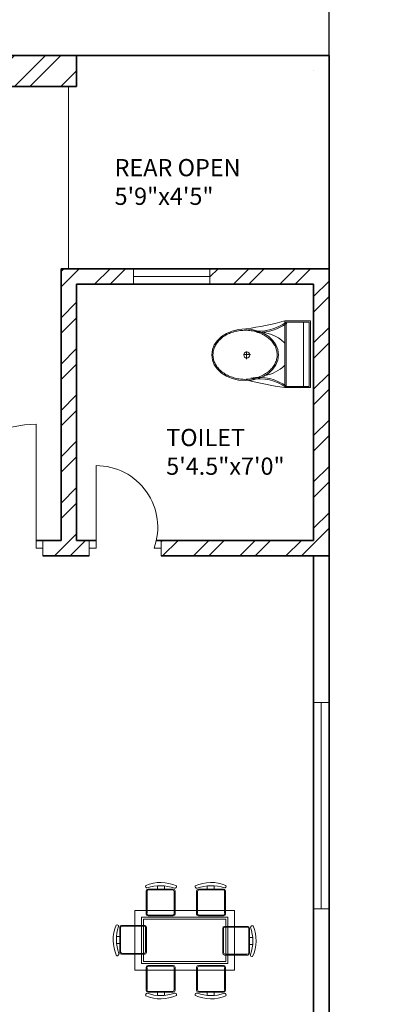
# Model space of a CAD drawing. Units: inches. Extents: x 1850 to 3445, y 1558 to 2756.
# Tile 4 of 13: x 2195 to 2304, y 1940 to 2227. Entities that reach past the tile are written whole.
import ezdxf

# ---------------------------------------------------------------- set-up
doc = ezdxf.new("R2010")
doc.units = ezdxf.units.IN
for name, color, linetype, lineweight in [('A-ANNO-DIMS', 2, 'Continuous', 18), ('A-AREA-IDEN', 7, 'Continuous', 18), ('A-DOOR', 3, 'Continuous', 18), ('A-FLOR-FIXT', 9, 'Continuous', 18), ('A-FURN', 8, 'Continuous', 13), ('A-GLAZ', 4, 'Continuous', 18), ('A-WALL', 7, 'Continuous', 35), ('A-WALL-PATT', 252, 'Continuous', 13)]:
    doc.layers.add(name, color=color, linetype=linetype, lineweight=lineweight)
doc.styles.get("Standard").update_dxf_attribs({"font": 'arial.ttf'})
doc.dimstyles.get("Standard").update_dxf_attribs({"dimtxt": 0.18, "dimasz": 0.18, "dimexe": 0.18, "dimexo": 0.0625, "dimgap": 0.09, "dimtad": 0, "dimtih": 1, "dimtoh": 1, "dimdec": 4, "dimzin": 0, "dimdsep": 46, "dimtxsty": 'Standard', "dimcen": 0.09, "dimadec": 0, "dimazin": 0, "dimtfac": 1, "dimtdec": 4, "dimtofl": 0, "dimtmove": 0, "dimatfit": 3, "dimfxl": 1, "dimtolj": 1, "dimtzin": 0, "dimarcsym": 0})

# ---------------------------------------------------------------- blocks, each defined once
blk = doc.blocks.new('A$C31115884')
for p, q in [((283.1, 497.7), (223.4, 497.7)), ((257.5, 466.4), (257.5, 523.2)), ((0, 200), (0, 0)), ((520, 200), (0, 200)), ((10, 190), (10, 10)), ((510, 190), (10, 190)), ((510, 10), (510, 190)), ((520, 0), (520, 200)), ((510, 54.5), (0, 54.5)), ((10, 10), (510, 10)), ((0, 0), (520, 0))]:
    blk.add_line(p, q)
blk.add_circle((255.6, 496.4), 23.6)
for centre, radius, start, end in [((2777.7, -204.6), 2807, 165.4549, 171.71327), ((-294.5, 403.3), 364.7, 324.20913, 9.34987), ((-294.5, 403.3), 374.7, 324.20913, 9.34987), ((805.8, 403.3), 364.7, 170.65013, 215.79087), ((3237, 905), 2807, 188.28673, 194.5451), ((139.5, 406.2), 293.5, 315.84364, 2.65635), ((805.8, 403.3), 374.7, 179.20365, 215.79087), ((383.6, 406.2), 293.5, 190.27735, 224.15636)]:
    blk.add_arc(centre, radius, start, end)
blk.add_ellipse((256.2, 509.9), major_axis=(0, -260.7), ratio=0.772727)
blk.add_open_spline([(256.2, 259.2), (263.1, 259.2), (270, 259.7), (287.8, 262.3), (298.7, 265.1), (319.9, 273.1), (330.2, 278.4), (350.1, 291.1), (359.7, 298.7), (377.7, 315.9), (386.2, 325.5), (401.7, 346.6), (408.8, 358.1), (421.3, 382.5), (426.8, 395.5), (435.9, 422.4), (439.5, 436.4), (444.8, 465.1), (446.5, 479.7), (447.9, 509.2), (447.6, 524), (445, 553.3), (442.7, 567.8), (436.3, 596), (432.1, 609.7), (421.9, 636), (416, 648.6), (402.5, 672.1), (395, 683), (378.6, 703), (369.8, 712.1), (351.1, 728), (341.3, 734.8), (320.9, 746.2), (310.4, 750.7), (288.9, 757.3), (278, 759.4), (256, 761), (245, 760.6), (223.1, 757.2), (212.3, 754.3), (191.1, 746.1), (180.8, 740.7), (160.9, 727.8), (151.4, 720.1), (133.5, 702.7), (125.1, 693), (109.6, 671.7), (102.6, 660.2), (90.2, 635.7), (84.9, 622.7), (76, 595.6), (72.4, 581.6), (67.2, 552.9), (65.6, 538.2), (64.4, 508.8), (64.8, 494), (67.5, 464.7), (69.9, 450.2), (76.6, 422), (80.8, 408.3), (91.1, 382.2), (97.2, 369.7), (110.8, 346.3), (118.4, 335.4), (134.8, 315.6), (143.7, 306.7), (162.4, 290.9), (172.3, 284.2), (192.8, 273), (203.3, 268.6), (224.8, 262.2), (235.8, 260.2), (249.9, 259.3), (253, 259.2), (256.2, 259.2)], degree=3, knots=[0, 0, 0, 0, 0.110105, 0.110105, 0.285049, 0.285049, 0.459994, 0.459994, 0.634938, 0.634938, 0.809882, 0.809882, 0.984827, 0.984827, 1.159771, 1.159771, 1.334715, 1.334715, 1.50966, 1.50966, 1.684604, 1.684604, 1.859549, 1.859549, 2.034493, 2.034493, 2.209437, 2.209437, 2.384382, 2.384382, 2.559326, 2.559326, 2.73427, 2.73427, 2.909215, 2.909215, 3.084159, 3.084159, 3.259103, 3.259103, 3.434048, 3.434048, 3.608992, 3.608992, 3.783936, 3.783936, 3.958881, 3.958881, 4.133825, 4.133825, 4.30877, 4.30877, 4.483714, 4.483714, 4.658658, 4.658658, 4.833603, 4.833603, 5.008547, 5.008547, 5.183491, 5.183491, 5.358436, 5.358436, 5.53338, 5.53338, 5.708324, 5.708324, 5.883269, 5.883269, 6.058213, 6.058213, 6.233158, 6.233158, 6.283185, 6.283185, 6.283185, 6.283185])
blk = doc.blocks.new('WIN-60-W4_5')
for p, q in [((0, 60), (4.5, 60)), ((4.5, 60), (2.25, 60)), ((2.25, 60), (2.25, 0)), ((2.25, 0), (0, 0)), ((0, 0), (4.5, 0))]:
    blk.add_line(p, q)
blk = doc.blocks.new('WIN-BATH-GROUND')
for p, q in [((0, 0), (0, 4.5)), ((22.27, 2.25), (22.27, 4.5)), ((22.27, 4.5), (22.27, 0)), ((0, 2.25), (22.27, 2.25))]:
    blk.add_line(p, q)
blk = doc.blocks.new('DOOR-BATH-GROUND')
for p, q in [((2, 2.25), (2, 26.25)), ((0, 4.5), (0, 0)), ((20.9, 4.5), (20.9, 0)), ((0, 0), (0, 2.25)), ((0, 2.25), (2, 2.25)), ((20.9, 2.25), (18.9, 2.25)), ((20.9, 0), (20.9, 2.25))]:
    blk.add_line(p, q)
blk.add_arc((2, 8.3), 17.95, 340.2941, 90)
blk = doc.blocks.new('DOOR-BED-GROUND')
for p, q in [((31.38, 2.25), (31.38, 38.25)), ((0, 4.5), (0, 0)), ((33.38, 4.5), (33.38, 0)), ((0, 0), (0, 2.25)), ((0, 2.25), (2, 2.25)), ((33.38, 2.25), (31.38, 2.25)), ((33.38, 0), (33.38, 2.25))]:
    blk.add_line(p, q)
blk.add_arc((31.38, 8.26), 29.99, 90, 191.5706)
blk = doc.blocks.new('*D80')
at = {"layer": 'A-ANNO-DIMS', "color": 0, "lineweight": -2, "transparency": 16777216}
for p, q in [((2040.27, 2216.25), (2040.27, 2244.61)), ((2040.45, 2244.43), (2162.48, 2244.43)), ((2285.09, 2244.43), (2163.06, 2244.43)), ((2285.27, 2216.25), (2285.27, 2244.61))]:
    blk.add_line(p, q, dxfattribs=at)
at = {"layer": 'A-ANNO-DIMS', "color": 0, "transparency": 16777216}
for points in [[(2040.45, 2244.46), (2040.45, 2244.4), (2040.27, 2244.43)], [(2285.09, 2244.46), (2285.09, 2244.4), (2285.27, 2244.43)]]:
    blk.add_solid(points, dxfattribs=at)
at = {"layer": 'Defpoints', "color": 0, "transparency": 16777216}
for p in [(2285.27, 2244.43), (2040.27, 2216.18), (2285.27, 2216.18)]:
    blk.add_point(p, dxfattribs=at)
at = {"layer": 'A-ANNO-DIMS', "color": 0, "transparency": 16777216, "insert": (2162.77, 2244.43), "char_height": 0.18, "attachment_point": 5}
blk.add_mtext('\\A1;245', dxfattribs=at)

msp = doc.modelspace()

# ---------------------------------------------------------------- hatches: boundary and pattern name
at = {"layer": 'A-WALL-PATT'}
h = msp.add_hatch(dxfattribs=at)
h.set_pattern_fill('ANSI32', color=256)
h.paths.add_polyline_path([(2519.5556, 1907.3936), (2523.9987, 1907.3936), (2523.9987, 1916.3936), (2519.5556, 1916.3936), (2515.0556, 1916.3936), (2510.5556, 1916.3936), (2510.5556, 1907.3936), (2515.0556, 1907.3936), (2515.0556, 1742.1843), (2515.0556, 1737.6843), (2596.0556, 1737.6843), (2596.0556, 1976.4962), (2591.5556, 1976.4962), (2591.5556, 1916.3936), (2561.2666, 1916.3936), (2561.2666, 1907.3936), (2591.5556, 1907.3936), (2591.5556, 1746.6843), (2519.5556, 1746.6843)])
h.paths.add_polyline_path([(2076.6481, 2211.6843), (2076.6481, 2216.1843), (2040.2715, 2216.1843), (2040.2715, 2175.83), (2044.7715, 2175.83), (2049.2715, 2175.83), (2049.2715, 2207.1843), (2076.6481, 2207.1843)])
h.paths.add_polyline_path([(2211.7715, 2216.1843), (2136.6481, 2216.1843), (2136.6481, 2207.1843), (2211.7715, 2207.1843)])
h.paths.add_polyline_path([(2285.2715, 2154.1843), (2250.6169, 2154.1843), (2250.6169, 2149.6843), (2280.7715, 2149.6843), (2280.7715, 2075.1843), (2236.3632, 2075.1843), (2236.3632, 2070.6843), (2285.2715, 2070.6843)])
h.paths.add_polyline_path([(2228.3485, 2154.1843), (2207.2715, 2154.1843), (2207.2715, 2075.1843), (2201.9819, 2075.1843), (2201.9819, 2070.6843), (2215.4663, 2070.6843), (2215.4663, 2072.9343), (2215.4663, 2075.1843), (2211.7715, 2075.1843), (2211.7715, 2149.6843), (2228.3485, 2149.6843)])
h.paths.add_polyline_path([(2049.2715, 2115.83), (2040.2715, 2115.83), (2040.2715, 2042.8465), (2049.2715, 2042.8465), (2049.2715, 2070.6843), (2168.6057, 2070.6843), (2168.6057, 2072.9343), (2168.6057, 2075.1843), (2049.2715, 2075.1843)])
h.paths.add_polyline_path([(2049.2715, 1982.8465), (2040.2715, 1982.8465), (2040.2715, 1910.2175), (2060.9481, 1910.2175), (2060.9481, 1914.7175), (2060.9481, 1919.2175), (2049.2715, 1919.2175)])
h.paths.add_polyline_path([(2132.4938, 1919.2175), (2108.9481, 1919.2175), (2108.9481, 1910.2175), (2132.4938, 1910.2175), (2132.4938, 1914.6749)])
h.paths.add_polyline_path([(2178.7715, 1938.6843), (2169.7715, 1938.6843), (2169.7715, 1919.2175), (2163.687, 1919.2175), (2163.687, 1910.2175), (2169.7715, 1910.2175), (2169.7715, 1854.6843), (2169.7715, 1845.6843), (2196.1287, 1845.6843), (2196.1287, 1850.1843), (2196.1287, 1854.6843), (2178.7715, 1854.6843)])
h.paths.add_polyline_path([(2049.2715, 1910.2175), (2040.2715, 1910.2175), (2040.2715, 1745.6843), (2049.2715, 1745.6843)])
h.paths.add_polyline_path([(2146.8861, 1766.7204), (2159.0894, 1766.7204), (2159.0894, 1777.0239), (2146.8861, 1777.0239)], flags=9)
h.paths.add_polyline_path([(2183.4664, 1798.4016), (2226.7338, 1798.4016), (2226.7338, 1817.0589), (2183.4664, 1817.0589)], flags=9)
h.paths.add_polyline_path([(2070.863, 1867.537), (2109.9796, 1867.537), (2109.9796, 1886.1943), (2070.863, 1886.1943)], flags=9)

# ---------------------------------------------------------------- linework, layer by layer
at = {"layer": 'A-FURN'}
for points in [[(2232.3545, 1974.0971, -0.17580919), (2240.2562, 1974.0373, 0.57839206), (2240.8548, 1974.6955, 0.21452438), (2231.9355, 1974.8152, 0.55201397), (2232.3545, 1974.0971, -0.06507904)], [(2232.3545, 1974.0968, -0.17580919), (2240.2562, 1974.037, 0.57839206), (2240.8548, 1974.6952, 0.21452438), (2231.9355, 1974.8149, 0.55201397), (2232.3545, 1974.0968, -0.06507904)], [(2246.9084, 1974.0373, -0.57839206), (2246.3098, 1974.6955, -0.21452438), (2255.2292, 1974.8152, -0.55201397), (2254.8101, 1974.0971, 0.1758092), (2246.9084, 1974.0373)], [(2246.9084, 1974.037, -0.57839206), (2246.3098, 1974.6952, -0.21452438), (2255.2292, 1974.8149, -0.55201397), (2254.8101, 1974.0968, 0.1758092), (2246.9084, 1974.037)], [(2239.921, 1973.78), (2232.5853, 1973.78, 0.41421356), (2232.0721, 1973.2668), (2232.0721, 1966.5217, 0.41421356), (2232.5853, 1966.0085), (2239.921, 1966.0085, 0.41421356), (2240.4342, 1966.5217), (2240.4342, 1973.2668, 0.41421356), (2239.921, 1973.78)], [(2239.921, 1973.7797), (2232.5853, 1973.7797, 0.41421356), (2232.0721, 1973.2665), (2232.0721, 1966.5214, 0.41421356), (2232.5853, 1966.0082), (2239.921, 1966.0082, 0.41421356), (2240.4342, 1966.5214), (2240.4342, 1973.2665, 0.41421356), (2239.921, 1973.7797)], [(2237.3443, 1973.78), (2237.3443, 1974.7077, -0.06475861)], [(2237.3443, 1973.7797), (2237.3443, 1974.7074, -0.06475861)], [(2254.5793, 1973.78, -0.41421356), (2255.0925, 1973.2668), (2255.0925, 1966.5217, -0.41421356), (2254.5793, 1966.0085), (2247.2437, 1966.0085, -0.41421356), (2246.7304, 1966.5217), (2246.7304, 1973.2668, -0.41421356), (2247.2437, 1973.78), (2254.5793, 1973.78)], [(2254.5793, 1973.7797, -0.41421356), (2255.0926, 1973.2665), (2255.0926, 1966.5214, -0.41421356), (2254.5793, 1966.0082), (2247.2437, 1966.0082, -0.41421356), (2246.7305, 1966.5214), (2246.7305, 1973.2665, -0.41421356), (2247.2437, 1973.7797), (2254.5793, 1973.7797)], [(2249.8203, 1973.78), (2249.8203, 1974.7077, 0.06475861)], [(2249.8203, 1973.7797), (2249.8203, 1974.7074, 0.06475861)], [(2224.0878, 1955.0157, -0.57839206), (2223.4296, 1954.4171, -0.21452438), (2223.3099, 1963.3364, -0.55201397), (2224.028, 1962.9174, 0.17580937), (2224.0878, 1955.0157)], [(2224.0878, 1955.0154, -0.57839206), (2223.4296, 1954.4168, -0.21452438), (2223.3099, 1963.3361, -0.55201397), (2224.028, 1962.9171, 0.17580937), (2224.0878, 1955.0154)], [(2224.3451, 1962.6866, -0.41421356), (2224.8583, 1963.1998), (2231.6033, 1963.1998, -0.41421356), (2232.1165, 1962.6866), (2232.1165, 1955.3509, -0.41421356), (2231.6033, 1954.8377), (2224.8583, 1954.8377, -0.41421356), (2224.3451, 1955.3509), (2224.3451, 1962.6866)], [(2224.3451, 1962.6863, -0.41421356), (2224.8583, 1963.1995), (2231.6033, 1963.1995, -0.41421356), (2232.1166, 1962.6863), (2232.1166, 1955.3506, -0.41421356), (2231.6033, 1954.8374), (2224.8583, 1954.8374, -0.41421356), (2224.3451, 1955.3506), (2224.3451, 1962.6863)], [(2262.1204, 1962.4354, 0.41421356), (2261.6072, 1962.9486), (2254.8622, 1962.9486, 0.41421356), (2254.349, 1962.4354), (2254.349, 1955.0997, 0.41421356), (2254.8622, 1954.5865), (2261.6072, 1954.5865, 0.41421356), (2262.1204, 1955.0997), (2262.1204, 1962.4354)], [(2262.1204, 1962.4351, 0.41421356), (2261.6072, 1962.9483), (2254.8622, 1962.9483, 0.41421356), (2254.349, 1962.4351), (2254.349, 1955.0994, 0.41421356), (2254.8622, 1954.5862), (2261.6072, 1954.5862, 0.41421356), (2262.1204, 1955.0994), (2262.1204, 1962.4351)], [(2262.4375, 1962.6662, -0.17580919), (2262.3777, 1954.7645, 0.57839206), (2263.0359, 1954.1658, 0.21452438), (2263.1556, 1963.0852, 0.55201397), (2262.4375, 1962.6662, -0.06507904)], [(2262.4375, 1962.6659, -0.17580919), (2262.3777, 1954.7642, 0.57839206), (2263.0359, 1954.1655, 0.21452438), (2263.1556, 1963.0849, 0.55201397), (2262.4375, 1962.6659, -0.06507904)], [(2224.3451, 1957.9276), (2223.4174, 1957.9276, 0.06475861)], [(2224.3451, 1957.9273), (2223.4174, 1957.9273, 0.06475861)], [(2262.1204, 1957.6764), (2263.0481, 1957.6764, -0.06475861)], [(2262.1204, 1957.676), (2263.0481, 1957.676, -0.06475861)], [(2239.921, 1943.7967), (2232.5853, 1943.7967, -0.41421356), (2232.0721, 1944.31), (2232.0721, 1951.055, -0.41421356), (2232.5853, 1951.5682), (2239.921, 1951.5682, -0.41421356), (2240.4342, 1951.055), (2240.4342, 1944.31, -0.41421356), (2239.921, 1943.7967)], [(2239.921, 1943.7964), (2232.5853, 1943.7964, -0.41421356), (2232.0721, 1944.3097), (2232.0721, 1951.0547, -0.41421356), (2232.5853, 1951.5679), (2239.921, 1951.5679, -0.41421356), (2240.4342, 1951.0547), (2240.4342, 1944.3097, -0.41421356), (2239.921, 1943.7964)], [(2254.5793, 1943.7967, 0.41421356), (2255.0925, 1944.31), (2255.0925, 1951.055, 0.41421356), (2254.5793, 1951.5682), (2247.2437, 1951.5682, 0.41421356), (2246.7304, 1951.055), (2246.7304, 1944.31, 0.41421356), (2247.2437, 1943.7967), (2254.5793, 1943.7967)], [(2254.5793, 1943.7964, 0.41421356), (2255.0926, 1944.3097), (2255.0926, 1951.0547, 0.41421356), (2254.5793, 1951.5679), (2247.2437, 1951.5679, 0.41421356), (2246.7305, 1951.0547), (2246.7305, 1944.3097, 0.41421356), (2247.2437, 1943.7964), (2254.5793, 1943.7964)], [(2240.2562, 1943.5394, -0.57839206), (2240.8548, 1942.8812, -0.21452438), (2231.9355, 1942.7615, -0.55201397), (2232.3545, 1943.4796, 0.17580929), (2240.2562, 1943.5394)], [(2240.2562, 1943.5391, -0.57839206), (2240.8548, 1942.8809, -0.21452438), (2231.9355, 1942.7612, -0.55201397), (2232.3545, 1943.4793, 0.17580929), (2240.2562, 1943.5391)], [(2237.3443, 1943.7967), (2237.3443, 1942.869, 0.06475861)], [(2237.3443, 1943.7964), (2237.3443, 1942.8687, 0.06475861)], [(2254.8101, 1943.4796, -0.17580928), (2246.9084, 1943.5394, 0.57839206), (2246.3098, 1942.8812, 0.21452438), (2255.2292, 1942.7615, 0.55201397), (2254.8101, 1943.4796, -0.06507904)], [(2254.8101, 1943.4793, -0.17580928), (2246.9084, 1943.5391, 0.57839206), (2246.3098, 1942.8809, 0.21452438), (2255.2292, 1942.7612, 0.55201397), (2254.8101, 1943.4793, -0.06507904)], [(2249.8203, 1943.7967), (2249.8203, 1942.869, -0.06475861)], [(2249.8203, 1943.7964), (2249.8203, 1942.8687, -0.06475861)]]:
    msp.add_lwpolyline(points, format="xyb", dxfattribs=at)
for points in [[(2232.5884, 1973.5488), (2239.6898, 1973.5488, -0.41421356), (2240.203, 1973.0356), (2240.203, 1966.753, -0.41421356), (2239.6898, 1966.2397), (2232.5884, 1966.2397, -0.51206948), (2232.3033, 1966.753), (2232.3033, 1973.0356, -0.51206948)], [(2232.5884, 1973.5485), (2239.6898, 1973.5485, -0.41421356), (2240.203, 1973.0352), (2240.203, 1966.7526, -0.41421356), (2239.6898, 1966.2394), (2232.5884, 1966.2394, -0.51206948), (2232.3033, 1966.7526), (2232.3033, 1973.0352, -0.51206948)], [(2254.5762, 1973.5488), (2247.4749, 1973.5488, 0.41421356), (2246.9617, 1973.0356), (2246.9617, 1966.753, 0.41421356), (2247.4749, 1966.2397), (2254.5762, 1966.2397, 0.51206948), (2254.8613, 1966.753), (2254.8613, 1973.0356, 0.51206948)], [(2254.5762, 1973.5485), (2247.4749, 1973.5485, 0.41421356), (2246.9617, 1973.0352), (2246.9617, 1966.7526, 0.41421356), (2247.4749, 1966.2394), (2254.5762, 1966.2394, 0.51206948), (2254.8614, 1966.7526), (2254.8614, 1973.0352, 0.51206948)], [(2224.5763, 1962.6835), (2224.5763, 1955.5821, 0.41421356), (2225.0895, 1955.0689), (2231.3721, 1955.0689, 0.41421356), (2231.8853, 1955.5821), (2231.8853, 1962.6835, 0.51206948), (2231.3721, 1962.9686), (2225.0895, 1962.9686, 0.51206948)], [(2224.5763, 1962.6832), (2224.5763, 1955.5818, 0.41421356), (2225.0895, 1955.0686), (2231.3721, 1955.0686, 0.41421356), (2231.8854, 1955.5818), (2231.8854, 1962.6832, 0.51206948), (2231.3721, 1962.9683), (2225.0895, 1962.9683, 0.51206948)], [(2261.8892, 1962.4323), (2261.8892, 1955.3309, -0.41421356), (2261.376, 1954.8177), (2255.0934, 1954.8177, -0.41421356), (2254.5802, 1955.3309), (2254.5802, 1962.4323, -0.51206948), (2255.0934, 1962.7174), (2261.376, 1962.7174, -0.51206948)], [(2261.8892, 1962.432), (2261.8892, 1955.3306, -0.41421356), (2261.376, 1954.8174), (2255.0934, 1954.8174, -0.41421356), (2254.5802, 1955.3306), (2254.5802, 1962.432, -0.51206948), (2255.0934, 1962.7171), (2261.376, 1962.7171, -0.51206948)], [(2232.5884, 1944.028), (2239.6898, 1944.028, 0.41421356), (2240.203, 1944.5412), (2240.203, 1950.8238, 0.41421356), (2239.6898, 1951.337), (2232.5884, 1951.337, 0.51206948), (2232.3033, 1950.8238), (2232.3033, 1944.5412, 0.51206948)], [(2232.5884, 1944.0276), (2239.6898, 1944.0276, 0.41421356), (2240.203, 1944.5409), (2240.203, 1950.8235, 0.41421356), (2239.6898, 1951.3367), (2232.5884, 1951.3367, 0.51206948), (2232.3033, 1950.8235), (2232.3033, 1944.5409, 0.51206948)], [(2254.5762, 1944.028), (2247.4749, 1944.028, -0.41421356), (2246.9617, 1944.5412), (2246.9617, 1950.8238, -0.41421356), (2247.4749, 1951.337), (2254.5762, 1951.337, -0.51206948), (2254.8613, 1950.8238), (2254.8613, 1944.5412, -0.51206948)], [(2254.5762, 1944.0276), (2247.4749, 1944.0276, -0.41421356), (2246.9617, 1944.5409), (2246.9617, 1950.8235, -0.41421356), (2247.4749, 1951.3367), (2254.5762, 1951.3367, -0.51206948), (2254.8614, 1950.8235), (2254.8614, 1944.5409, -0.51206948)]]:
    msp.add_lwpolyline(points, format="xyb", close=True, dxfattribs=at)
for points in [[(2235.291, 1974.7246), (2235.291, 1973.78)], [(2235.291, 1974.7243), (2235.291, 1973.7797)], [(2251.8737, 1974.7246), (2251.8737, 1973.78)], [(2251.8737, 1974.7243), (2251.8737, 1973.7797)], [(2223.4005, 1959.9809), (2224.3451, 1959.9809)], [(2223.4005, 1959.9806), (2224.3451, 1959.9806)], [(2263.065, 1959.7297), (2262.1204, 1959.7297)], [(2263.065, 1959.7294), (2262.1204, 1959.7294)], [(2235.291, 1942.8521), (2235.291, 1943.7967)], [(2235.291, 1942.8518), (2235.291, 1943.7964)], [(2251.8737, 1942.8521), (2251.8737, 1943.7967)], [(2251.8737, 1942.8518), (2251.8737, 1943.7964)]]:
    msp.add_lwpolyline(points, dxfattribs=at)
for points in [[(2228.7662, 1967.5848), (2257.7769, 1967.5848), (2257.7769, 1950.1784), (2228.7662, 1950.1784)], [(2228.7662, 1967.5845), (2257.7769, 1967.5845), (2257.7769, 1950.1781), (2228.7662, 1950.1781)], [(2230.7002, 1965.6508), (2255.8429, 1965.6508), (2255.8429, 1952.1124), (2230.7002, 1952.1124)], [(2230.7002, 1965.6504), (2255.8429, 1965.6504), (2255.8429, 1952.1121), (2230.7002, 1952.1121)], [(2231.2804, 1965.0705), (2255.2627, 1965.0705), (2255.2627, 1952.6926), (2231.2804, 1952.6926)], [(2231.2805, 1965.0702), (2255.2627, 1965.0702), (2255.2627, 1952.6923), (2231.2805, 1952.6923)]]:
    msp.add_lwpolyline(points, close=True, dxfattribs=at)
at = {"layer": 'A-GLAZ'}
msp.add_line((2209.4518, 2207.1843), (2209.4518, 2154.1843), dxfattribs=at)
at = {"layer": 'A-WALL'}
for p, q in [((2040.2715, 2216.1843), (2285.2715, 2216.1843)), ((2211.7715, 2216.1843), (2211.7715, 2207.1843)), ((2285.2715, 2207.1843), (2285.2715, 2216.1843)), ((2280.7444, 2211.8893), (2280.7444, 2211.8893)), ((2049.2715, 2207.1843), (2211.7715, 2207.1843)), ((2285.2715, 2207.1843), (2285.2715, 1745.6843)), ((2207.2715, 2154.1843), (2207.2715, 2075.1843)), ((2207.2715, 2154.1843), (2285.2715, 2154.1843)), ((2211.7715, 2149.6843), (2280.7715, 2149.6843)), ((2211.7715, 2149.6843), (2211.7715, 2075.1843)), ((2280.7715, 2149.6843), (2280.7715, 2075.1843)), ((2199.9819, 2075.1843), (2207.2715, 2075.1843)), ((2211.7715, 2075.1843), (2217.4663, 2075.1843)), ((2235.0071, 2075.1843), (2280.7715, 2075.1843)), ((2201.9819, 2070.6843), (2215.4663, 2070.6843)), ((2236.3632, 2070.6843), (2285.2715, 2070.6843)), ((2280.7715, 2070.6843), (2280.7715, 1854.6843))]:
    msp.add_line(p, q, dxfattribs=at)

# ---------------------------------------------------------------- block references
at = {"layer": 'A-DOOR'}
for name, p in [('DOOR-BED-GROUND', (2168.606, 2070.684)), ('DOOR-BATH-GROUND', (2215.466, 2070.684))]:
    msp.add_blockref(name, p, dxfattribs=at)
at = {"layer": 'A-FLOR-FIXT', "xscale": 0.0372717239612423, "yscale": 0.0372717239612423, "zscale": 0.0372717239612423, "rotation": 89.99999999999999}
msp.add_blockref('A$C31115884', (2279.8375, 2119.6), dxfattribs=at)
at = {"layer": 'A-GLAZ'}
for name, p in [('WIN-BATH-GROUND', (2228.349, 2149.684)), ('WIN-60-W4_5', (2280.771, 1968.032))]:
    msp.add_blockref(name, p, dxfattribs=at)

# ---------------------------------------------------------------- texts
at = {"layer": 'A-AREA-IDEN', "char_height": 5, "attachment_point": 1}
for s, width, insert in [('REAR OPEN\\P5\'9"x4\'5"', 99.200616, (2222.8413, 2186.0812)), ('TOILET\\P5\'4.5"x7\'0"', 96.193359, (2237.8692, 2107.5965))]:
    msp.add_mtext_dynamic_manual_height_columns(s, width=width, gutter_width=12.5, heights=[0], dxfattribs=dict(at, insert=insert))

# ---------------------------------------------------------------- dimensions: what is measured, and where the dimension line sits
at = {"layer": 'A-ANNO-DIMS'}
dim = msp.add_linear_dim(base=(2285.2715, 2244.4343), p1=(2040.2715, 2216.1843), p2=(2285.2715, 2216.1843), dimstyle='Standard', override={"dimdec": 0, "dimlfac": 1, "dimrnd": 0, "dimzin": 0, "dimdsep": 46, "dimlunit": 2}, dxfattribs=at)
dim.commit()
dim.dimension.update_dxf_attribs({"geometry": '*D80', "text_midpoint": (2162.7715, 2244.4343)})

doc.saveas('drawing.dxf')
